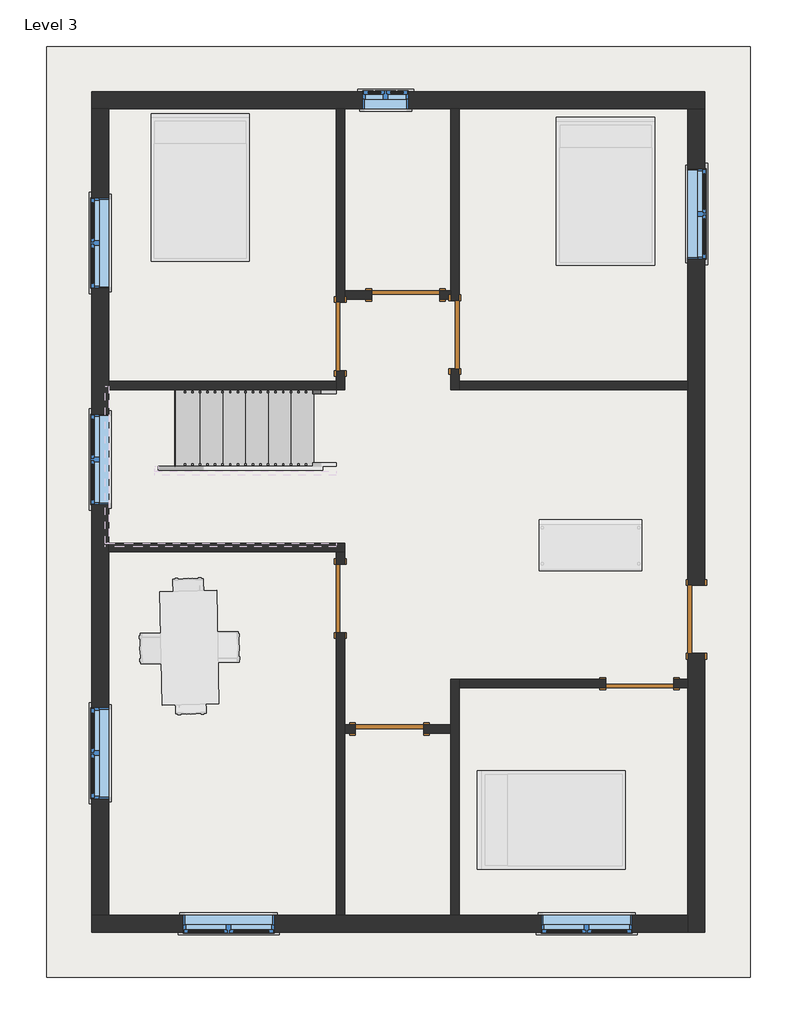
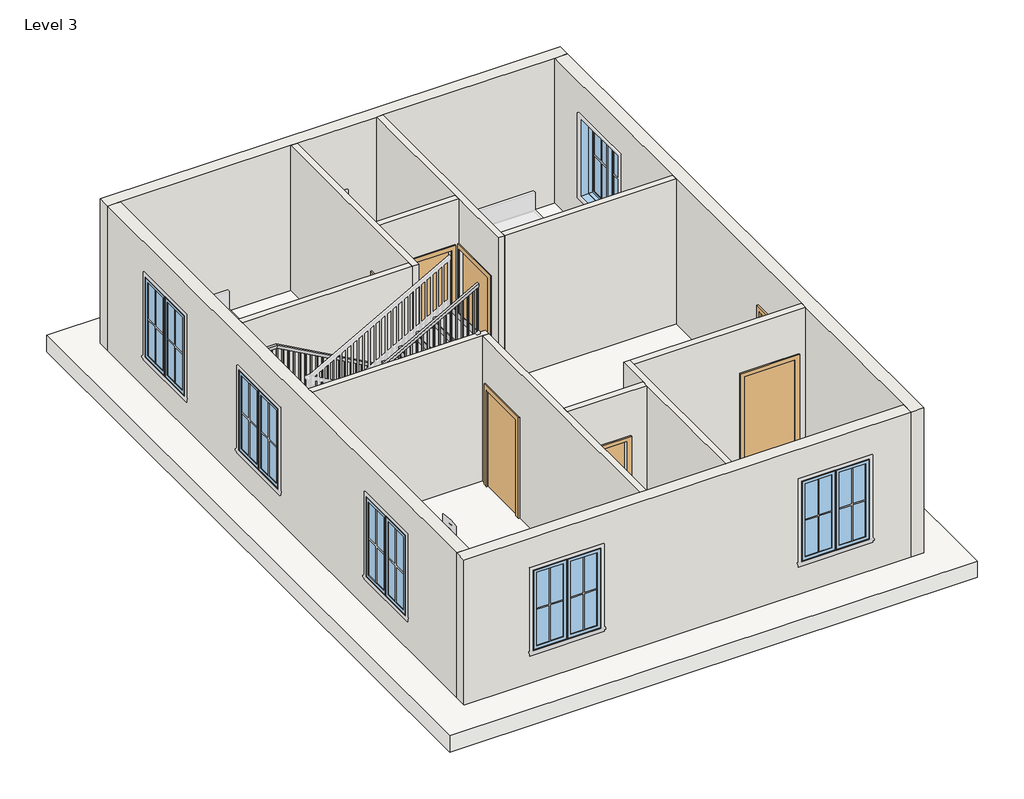
# One storey, part 1 of 2: 14 walls, 7 doors, 7 windows, 1 railing, 1 roof, 1 stair flight.
"""IFC4 building model written with IfcOpenShell, lengths in millimetres."""

from ifc_helpers import new_model, si_unit, frame, origin, place, context, project, spatial, polyline, outline, extrude, faceted_brep, transform, mapped, element, save
from components import door_e5f9f3c4, door_305aa2a5, door_a90ba1ad, stair_flight_67f7f0a7, window_c417fced, window_8377141f

model = new_model("IFC4")

# Units and contexts
model_context = context("Model", 3, world=origin())
ifc_project = project(units=[si_unit("LENGTHUNIT", "METRE", prefix="MILLI")], contexts=[model_context])

# Site, building, storey
site = spatial("IfcSite", under=ifc_project)
building = spatial("IfcBuilding", under=site)
storey = spatial("IfcBuildingStorey", under=building, Name="Level 3", Elevation=6096.0)

# Doors
placement = place(None, origin())
door_shape = door_e5f9f3c4(model_context)
element("IfcDoor", 1, ObjectType="Single-Flush : 36\" x 84\"", at=placement, inside=storey, context=model_context, shape_type="MappedRepresentation", body=[
    mapped(door_shape, transform((5226.05, 11245.85, 6096.0), x_axis=(1.0, 0.0, 0.0), y_axis=(0.0, 1.0, 0.0), z_axis=(0.0, 0.0, 1.0))),
])
element("IfcDoor", 2, ObjectType="Single-Flush : 36\" x 84\"", at=placement, inside=storey, context=model_context, shape_type="MappedRepresentation", body=[
    mapped(door_shape, transform((5886.45, 10712.45, 6096.0), x_axis=(0.0, -1.0, 0.0), y_axis=(1.0, 0.0, 0.0), z_axis=(0.0, 0.0, 1.0))),
])
door_2_shape = door_305aa2a5(model_context)
element("IfcDoor", 3, ObjectType="Single-Flush : 36\" x 84\"", at=placement, inside=storey, context=model_context, shape_type="MappedRepresentation", body=[
    mapped(door_2_shape, transform((4349.75, 10687.05, 6096.0), x_axis=(0.0, -1.0, 0.0), y_axis=(1.0, 0.0, 0.0), z_axis=(0.0, 0.0, 1.0))),
])
element("IfcDoor", 4, ObjectType="Single-Flush : 36\" x 84\"", at=placement, inside=storey, context=model_context, shape_type="MappedRepresentation", body=[
    mapped(door_2_shape, transform((8369.3, 6026.15, 6096.0), x_axis=(1.0, 0.0, 0.0), y_axis=(0.0, 1.0, 0.0), z_axis=(0.0, 0.0, 1.0))),
])
element("IfcDoor", 5, ObjectType="Single-Flush : 36\" x 84\"", at=placement, inside=storey, context=model_context, shape_type="MappedRepresentation", body=[
    mapped(door_2_shape, transform((5010.15, 5416.55, 6096.0), x_axis=(-1.0, 0.0, 0.0), y_axis=(0.0, -1.0, 0.0), z_axis=(0.0, 0.0, 1.0))),
])
element("IfcDoor", 6, ObjectType="Single-Flush : 36\" x 84\"", at=placement, inside=storey, context=model_context, shape_type="MappedRepresentation", body=[
    mapped(door_2_shape, transform((4349.75, 7169.15, 6096.0), x_axis=(0.0, -1.0, 0.0), y_axis=(1.0, 0.0, 0.0), z_axis=(0.0, 0.0, 1.0))),
])
door_3_shape = door_a90ba1ad(model_context)
element("IfcDoor", 7, ObjectType="Single-Flush : 36\" x 84\"", at=placement, inside=storey, context=model_context, shape_type="MappedRepresentation", body=[
    mapped(door_3_shape, transform((9131.3, 6889.75, 6096.0), x_axis=(0.0, -1.0, 0.0), y_axis=(1.0, 0.0, 0.0), z_axis=(0.0, 0.0, 1.0))),
])

# Railing
element("IfcRailing", 8, ObjectType="Handrail - Rectangular", at=placement, inside=storey, context=model_context, shape_type="SolidModel", body=[
    faceted_brep([(4295.1355783, 9918.7, 7179.7333333), (4295.1355783, 9918.7, 7121.620221), (4295.1355783, 9969.5, 7121.620221), (4295.1355783, 9969.5, 7179.7333333), (1856.7355783, 9918.7, 8534.4), (1843.5719761, 9918.7, 8483.6), (1843.5719761, 9969.5, 8483.6), (1856.7355783, 9969.5, 8534.4), (1295.4, 9918.7, 8534.4), (1295.4, 9918.7, 8483.6), (1244.6, 9969.5, 8483.6), (1244.6, 9969.5, 8534.4), (1295.4, 7962.9, 8534.4), (1295.4, 7962.9, 8483.6), (1244.6, 7912.1, 8483.6), (1244.6, 7912.1, 8534.4), (1551.9355783, 7962.9, 8534.4), (1565.0991806, 7962.9, 8483.6), (1565.0991806, 7912.1, 8483.6), (1551.9355783, 7912.1, 8534.4), (4295.1355783, 7962.9, 10058.4), (4295.1355783, 7912.1, 10058.4), (4295.1355783, 7912.1, 10000.2868876), (4295.1355783, 7962.9, 10000.2868876)], [[[0, 1, 2, 3]], [[1, 0, 4, 5]], [[2, 1, 5, 6]], [[3, 2, 6, 7]], [[0, 3, 7, 4]], [[5, 4, 8, 9]], [[6, 5, 9, 10]], [[7, 6, 10, 11]], [[4, 7, 11, 8]], [[9, 8, 12, 13]], [[10, 9, 13, 14]], [[11, 10, 14, 15]], [[8, 11, 15, 12]], [[13, 12, 16, 17]], [[14, 13, 17, 18]], [[15, 14, 18, 19]], [[12, 15, 19, 16]], [[20, 21, 22, 23]], [[17, 16, 20, 23]], [[18, 17, 23, 22]], [[19, 18, 22, 21]], [[16, 19, 21, 20]]]),
    extrude(outline(polyline([(9961.8365664, 4225.925), (9951.253233, 4206.875), (8974.6666667, 4206.875), (8974.6666667, 4225.925), (9961.8365664, 4225.925)])), frame((0.0, 7927.975, 0.0), z_axis=(0.0, 1.0, 0.0), x_axis=(0.0, 0.0, 1.0)), (0.0, 0.0, 1.0), 19.05),
    extrude(outline(polyline([(9905.3921219, 4124.325), (9894.8087886, 4105.275), (8974.6666667, 4105.275), (8974.6666667, 4124.325), (9905.3921219, 4124.325)])), frame((0.0, 7927.975, 0.0), z_axis=(0.0, 1.0, 0.0), x_axis=(0.0, 0.0, 1.0)), (0.0, 0.0, 1.0), 19.05),
    extrude(outline(polyline([(9848.9476775, 4022.725), (9838.3643441, 4003.675), (8974.6666667, 4003.675), (8974.6666667, 4022.725), (9848.9476775, 4022.725)])), frame((0.0, 7927.975, 0.0), z_axis=(0.0, 1.0, 0.0), x_axis=(0.0, 0.0, 1.0)), (0.0, 0.0, 1.0), 19.05),
    extrude(outline(polyline([(9792.503233, 3921.125), (9781.9198997, 3902.075), (8805.3333333, 3902.075), (8805.3333333, 3921.125), (9792.503233, 3921.125)])), frame((0.0, 7927.975, 0.0), z_axis=(0.0, 1.0, 0.0), x_axis=(0.0, 0.0, 1.0)), (0.0, 0.0, 1.0), 19.05),
    extrude(outline(polyline([(9736.0587886, 3819.525), (9725.4754552, 3800.475), (8805.3333333, 3800.475), (8805.3333333, 3819.525), (9736.0587886, 3819.525)])), frame((0.0, 7927.975, 0.0), z_axis=(0.0, 1.0, 0.0), x_axis=(0.0, 0.0, 1.0)), (0.0, 0.0, 1.0), 19.05),
    extrude(outline(polyline([(9679.6143441, 3717.925), (9669.0310108, 3698.875), (8805.3333333, 3698.875), (8805.3333333, 3717.925), (9679.6143441, 3717.925)])), frame((0.0, 7927.975, 0.0), z_axis=(0.0, 1.0, 0.0), x_axis=(0.0, 0.0, 1.0)), (0.0, 0.0, 1.0), 19.05),
    extrude(outline(polyline([(9623.1698997, 3616.325), (9612.5865664, 3597.275), (8636.0, 3597.275), (8636.0, 3616.325), (9623.1698997, 3616.325)])), frame((0.0, 7927.975, 0.0), z_axis=(0.0, 1.0, 0.0), x_axis=(0.0, 0.0, 1.0)), (0.0, 0.0, 1.0), 19.05),
    extrude(outline(polyline([(9566.7254552, 3514.725), (9556.1421219, 3495.675), (8636.0, 3495.675), (8636.0, 3514.725), (9566.7254552, 3514.725)])), frame((0.0, 7927.975, 0.0), z_axis=(0.0, 1.0, 0.0), x_axis=(0.0, 0.0, 1.0)), (0.0, 0.0, 1.0), 19.05),
    extrude(outline(polyline([(9510.2810108, 3413.125), (9499.6976775, 3394.075), (8636.0, 3394.075), (8636.0, 3413.125), (9510.2810108, 3413.125)])), frame((0.0, 7927.975, 0.0), z_axis=(0.0, 1.0, 0.0), x_axis=(0.0, 0.0, 1.0)), (0.0, 0.0, 1.0), 19.05),
    extrude(outline(polyline([(9453.8365664, 3311.525), (9443.253233, 3292.475), (8466.6666667, 3292.475), (8466.6666667, 3311.525), (9453.8365664, 3311.525)])), frame((0.0, 7927.975, 0.0), z_axis=(0.0, 1.0, 0.0), x_axis=(0.0, 0.0, 1.0)), (0.0, 0.0, 1.0), 19.05),
    extrude(outline(polyline([(9397.3921219, 3209.925), (9386.8087886, 3190.875), (8466.6666667, 3190.875), (8466.6666667, 3209.925), (9397.3921219, 3209.925)])), frame((0.0, 7927.975, 0.0), z_axis=(0.0, 1.0, 0.0), x_axis=(0.0, 0.0, 1.0)), (0.0, 0.0, 1.0), 19.05),
    extrude(outline(polyline([(9340.9476775, 3108.325), (9330.3643441, 3089.275), (8466.6666667, 3089.275), (8466.6666667, 3108.325), (9340.9476775, 3108.325)])), frame((0.0, 7927.975, 0.0), z_axis=(0.0, 1.0, 0.0), x_axis=(0.0, 0.0, 1.0)), (0.0, 0.0, 1.0), 19.05),
    extrude(outline(polyline([(9284.503233, 3006.725), (9273.9198997, 2987.675), (8297.3333333, 2987.675), (8297.3333333, 3006.725), (9284.503233, 3006.725)])), frame((0.0, 7927.975, 0.0), z_axis=(0.0, 1.0, 0.0), x_axis=(0.0, 0.0, 1.0)), (0.0, 0.0, 1.0), 19.05),
    extrude(outline(polyline([(9228.0587886, 2905.125), (9217.4754552, 2886.075), (8297.3333333, 2886.075), (8297.3333333, 2905.125), (9228.0587886, 2905.125)])), frame((0.0, 7927.975, 0.0), z_axis=(0.0, 1.0, 0.0), x_axis=(0.0, 0.0, 1.0)), (0.0, 0.0, 1.0), 19.05),
    extrude(outline(polyline([(9171.6143441, 2803.525), (9161.0310108, 2784.475), (8297.3333333, 2784.475), (8297.3333333, 2803.525), (9171.6143441, 2803.525)])), frame((0.0, 7927.975, 0.0), z_axis=(0.0, 1.0, 0.0), x_axis=(0.0, 0.0, 1.0)), (0.0, 0.0, 1.0), 19.05),
    extrude(outline(polyline([(9115.1698997, 2701.925), (9104.5865664, 2682.875), (8128.0, 2682.875), (8128.0, 2701.925), (9115.1698997, 2701.925)])), frame((0.0, 7927.975, 0.0), z_axis=(0.0, 1.0, 0.0), x_axis=(0.0, 0.0, 1.0)), (0.0, 0.0, 1.0), 19.05),
    extrude(outline(polyline([(9058.7254552, 2600.325), (9048.1421219, 2581.275), (8128.0, 2581.275), (8128.0, 2600.325), (9058.7254552, 2600.325)])), frame((0.0, 7927.975, 0.0), z_axis=(0.0, 1.0, 0.0), x_axis=(0.0, 0.0, 1.0)), (0.0, 0.0, 1.0), 19.05),
    extrude(outline(polyline([(9002.2810108, 2498.725), (8991.6976775, 2479.675), (8128.0, 2479.675), (8128.0, 2498.725), (9002.2810108, 2498.725)])), frame((0.0, 7927.975, 0.0), z_axis=(0.0, 1.0, 0.0), x_axis=(0.0, 0.0, 1.0)), (0.0, 0.0, 1.0), 19.05),
    extrude(outline(polyline([(8945.8365664, 2397.125), (8935.253233, 2378.075), (7958.6666667, 2378.075), (7958.6666667, 2397.125), (8945.8365664, 2397.125)])), frame((0.0, 7927.975, 0.0), z_axis=(0.0, 1.0, 0.0), x_axis=(0.0, 0.0, 1.0)), (0.0, 0.0, 1.0), 19.05),
    extrude(outline(polyline([(8889.3921219, 2295.525), (8878.8087886, 2276.475), (7958.6666667, 2276.475), (7958.6666667, 2295.525), (8889.3921219, 2295.525)])), frame((0.0, 7927.975, 0.0), z_axis=(0.0, 1.0, 0.0), x_axis=(0.0, 0.0, 1.0)), (0.0, 0.0, 1.0), 19.05),
    extrude(outline(polyline([(8832.9476775, 2193.925), (8822.3643441, 2174.875), (7958.6666667, 2174.875), (7958.6666667, 2193.925), (8832.9476775, 2193.925)])), frame((0.0, 7927.975, 0.0), z_axis=(0.0, 1.0, 0.0), x_axis=(0.0, 0.0, 1.0)), (0.0, 0.0, 1.0), 19.05),
    extrude(outline(polyline([(8776.503233, 2092.325), (8765.9198997, 2073.275), (7789.3333333, 2073.275), (7789.3333333, 2092.325), (8776.503233, 2092.325)])), frame((0.0, 7927.975, 0.0), z_axis=(0.0, 1.0, 0.0), x_axis=(0.0, 0.0, 1.0)), (0.0, 0.0, 1.0), 19.05),
    extrude(outline(polyline([(8720.0587886, 1990.725), (8709.4754552, 1971.675), (7789.3333333, 1971.675), (7789.3333333, 1990.725), (8720.0587886, 1990.725)])), frame((0.0, 7927.975, 0.0), z_axis=(0.0, 1.0, 0.0), x_axis=(0.0, 0.0, 1.0)), (0.0, 0.0, 1.0), 19.05),
    extrude(outline(polyline([(8663.6143441, 1889.125), (8653.0310108, 1870.075), (7789.3333333, 1870.075), (7789.3333333, 1889.125), (8663.6143441, 1889.125)])), frame((0.0, 7927.975, 0.0), z_axis=(0.0, 1.0, 0.0), x_axis=(0.0, 0.0, 1.0)), (0.0, 0.0, 1.0), 19.05),
    extrude(outline(polyline([(8607.1698997, 1787.525), (8596.5865664, 1768.475), (7620.0, 1768.475), (7620.0, 1787.525), (8607.1698997, 1787.525)])), frame((0.0, 7927.975, 0.0), z_axis=(0.0, 1.0, 0.0), x_axis=(0.0, 0.0, 1.0)), (0.0, 0.0, 1.0), 19.05),
    extrude(outline(polyline([(8550.7254552, 1685.925), (8540.1421219, 1666.875), (7620.0, 1666.875), (7620.0, 1685.925), (8550.7254552, 1685.925)])), frame((0.0, 7927.975, 0.0), z_axis=(0.0, 1.0, 0.0), x_axis=(0.0, 0.0, 1.0)), (0.0, 0.0, 1.0), 19.05),
    extrude(outline(polyline([(8494.2810108, 1584.325), (8483.6976775, 1565.275), (7620.0, 1565.275), (7620.0, 1584.325), (8494.2810108, 1584.325)])), frame((0.0, 7927.975, 0.0), z_axis=(0.0, 1.0, 0.0), x_axis=(0.0, 0.0, 1.0)), (0.0, 0.0, 1.0), 19.05),
    extrude(outline(polyline([(1463.675, 7927.975), (1463.675, 7947.025), (1482.725, 7947.025), (1482.725, 7927.975), (1463.675, 7927.975)])), frame((0.0, 0.0, 7620.0), z_axis=(0.0, 0.0, 1.0), x_axis=(1.0, 0.0, 0.0)), (0.0, 0.0, 1.0), 863.6),
    extrude(outline(polyline([(1362.075, 7927.975), (1362.075, 7947.025), (1381.125, 7947.025), (1381.125, 7927.975), (1362.075, 7927.975)])), frame((0.0, 0.0, 7620.0), z_axis=(0.0, 0.0, 1.0), x_axis=(1.0, 0.0, 0.0)), (0.0, 0.0, 1.0), 863.6),
    extrude(outline(polyline([(1260.475, 8023.225), (1279.525, 8023.225), (1279.525, 8004.175), (1260.475, 8004.175), (1260.475, 8023.225)])), frame((0.0, 0.0, 7620.0), z_axis=(0.0, 0.0, 1.0), x_axis=(1.0, 0.0, 0.0)), (0.0, 0.0, 1.0), 863.6),
    extrude(outline(polyline([(1260.475, 8124.825), (1279.525, 8124.825), (1279.525, 8105.775), (1260.475, 8105.775), (1260.475, 8124.825)])), frame((0.0, 0.0, 7620.0), z_axis=(0.0, 0.0, 1.0), x_axis=(1.0, 0.0, 0.0)), (0.0, 0.0, 1.0), 863.6),
    extrude(outline(polyline([(1260.475, 8226.425), (1279.525, 8226.425), (1279.525, 8207.375), (1260.475, 8207.375), (1260.475, 8226.425)])), frame((0.0, 0.0, 7620.0), z_axis=(0.0, 0.0, 1.0), x_axis=(1.0, 0.0, 0.0)), (0.0, 0.0, 1.0), 863.6),
    extrude(outline(polyline([(1260.475, 8328.025), (1279.525, 8328.025), (1279.525, 8308.975), (1260.475, 8308.975), (1260.475, 8328.025)])), frame((0.0, 0.0, 7620.0), z_axis=(0.0, 0.0, 1.0), x_axis=(1.0, 0.0, 0.0)), (0.0, 0.0, 1.0), 863.6),
    extrude(outline(polyline([(1260.475, 8429.625), (1279.525, 8429.625), (1279.525, 8410.575), (1260.475, 8410.575), (1260.475, 8429.625)])), frame((0.0, 0.0, 7620.0), z_axis=(0.0, 0.0, 1.0), x_axis=(1.0, 0.0, 0.0)), (0.0, 0.0, 1.0), 863.6),
    extrude(outline(polyline([(1260.475, 8531.225), (1279.525, 8531.225), (1279.525, 8512.175), (1260.475, 8512.175), (1260.475, 8531.225)])), frame((0.0, 0.0, 7620.0), z_axis=(0.0, 0.0, 1.0), x_axis=(1.0, 0.0, 0.0)), (0.0, 0.0, 1.0), 863.6),
    extrude(outline(polyline([(1260.475, 8632.825), (1279.525, 8632.825), (1279.525, 8613.775), (1260.475, 8613.775), (1260.475, 8632.825)])), frame((0.0, 0.0, 7620.0), z_axis=(0.0, 0.0, 1.0), x_axis=(1.0, 0.0, 0.0)), (0.0, 0.0, 1.0), 863.6),
    extrude(outline(polyline([(1260.475, 8734.425), (1279.525, 8734.425), (1279.525, 8715.375), (1260.475, 8715.375), (1260.475, 8734.425)])), frame((0.0, 0.0, 7620.0), z_axis=(0.0, 0.0, 1.0), x_axis=(1.0, 0.0, 0.0)), (0.0, 0.0, 1.0), 863.6),
    extrude(outline(polyline([(1260.475, 8836.025), (1279.525, 8836.025), (1279.525, 8816.975), (1260.475, 8816.975), (1260.475, 8836.025)])), frame((0.0, 0.0, 7620.0), z_axis=(0.0, 0.0, 1.0), x_axis=(1.0, 0.0, 0.0)), (0.0, 0.0, 1.0), 863.6),
    extrude(outline(polyline([(1260.475, 8937.625), (1279.525, 8937.625), (1279.525, 8918.575), (1260.475, 8918.575), (1260.475, 8937.625)])), frame((0.0, 0.0, 7620.0), z_axis=(0.0, 0.0, 1.0), x_axis=(1.0, 0.0, 0.0)), (0.0, 0.0, 1.0), 863.6),
    extrude(outline(polyline([(1260.475, 9039.225), (1279.525, 9039.225), (1279.525, 9020.175), (1260.475, 9020.175), (1260.475, 9039.225)])), frame((0.0, 0.0, 7620.0), z_axis=(0.0, 0.0, 1.0), x_axis=(1.0, 0.0, 0.0)), (0.0, 0.0, 1.0), 863.6),
    extrude(outline(polyline([(1260.475, 9140.825), (1279.525, 9140.825), (1279.525, 9121.775), (1260.475, 9121.775), (1260.475, 9140.825)])), frame((0.0, 0.0, 7620.0), z_axis=(0.0, 0.0, 1.0), x_axis=(1.0, 0.0, 0.0)), (0.0, 0.0, 1.0), 863.6),
    extrude(outline(polyline([(1260.475, 9242.425), (1279.525, 9242.425), (1279.525, 9223.375), (1260.475, 9223.375), (1260.475, 9242.425)])), frame((0.0, 0.0, 7620.0), z_axis=(0.0, 0.0, 1.0), x_axis=(1.0, 0.0, 0.0)), (0.0, 0.0, 1.0), 863.6),
    extrude(outline(polyline([(1260.475, 9344.025), (1279.525, 9344.025), (1279.525, 9324.975), (1260.475, 9324.975), (1260.475, 9344.025)])), frame((0.0, 0.0, 7620.0), z_axis=(0.0, 0.0, 1.0), x_axis=(1.0, 0.0, 0.0)), (0.0, 0.0, 1.0), 863.6),
    extrude(outline(polyline([(1260.475, 9445.625), (1279.525, 9445.625), (1279.525, 9426.575), (1260.475, 9426.575), (1260.475, 9445.625)])), frame((0.0, 0.0, 7620.0), z_axis=(0.0, 0.0, 1.0), x_axis=(1.0, 0.0, 0.0)), (0.0, 0.0, 1.0), 863.6),
    extrude(outline(polyline([(1260.475, 9547.225), (1279.525, 9547.225), (1279.525, 9528.175), (1260.475, 9528.175), (1260.475, 9547.225)])), frame((0.0, 0.0, 7620.0), z_axis=(0.0, 0.0, 1.0), x_axis=(1.0, 0.0, 0.0)), (0.0, 0.0, 1.0), 863.6),
    extrude(outline(polyline([(1260.475, 9648.825), (1279.525, 9648.825), (1279.525, 9629.775), (1260.475, 9629.775), (1260.475, 9648.825)])), frame((0.0, 0.0, 7620.0), z_axis=(0.0, 0.0, 1.0), x_axis=(1.0, 0.0, 0.0)), (0.0, 0.0, 1.0), 863.6),
    extrude(outline(polyline([(1260.475, 9750.425), (1279.525, 9750.425), (1279.525, 9731.375), (1260.475, 9731.375), (1260.475, 9750.425)])), frame((0.0, 0.0, 7620.0), z_axis=(0.0, 0.0, 1.0), x_axis=(1.0, 0.0, 0.0)), (0.0, 0.0, 1.0), 863.6),
    extrude(outline(polyline([(1260.475, 9852.025), (1279.525, 9852.025), (1279.525, 9832.975), (1260.475, 9832.975), (1260.475, 9852.025)])), frame((0.0, 0.0, 7620.0), z_axis=(0.0, 0.0, 1.0), x_axis=(1.0, 0.0, 0.0)), (0.0, 0.0, 1.0), 863.6),
    extrude(outline(polyline([(1358.2605783, 9953.625), (1358.2605783, 9934.575), (1339.2105783, 9934.575), (1339.2105783, 9953.625), (1358.2605783, 9953.625)])), frame((0.0, 0.0, 7620.0), z_axis=(0.0, 0.0, 1.0), x_axis=(1.0, 0.0, 0.0)), (0.0, 0.0, 1.0), 863.6),
    extrude(outline(polyline([(1459.8605783, 9953.625), (1459.8605783, 9934.575), (1440.8105783, 9934.575), (1440.8105783, 9953.625), (1459.8605783, 9953.625)])), frame((0.0, 0.0, 7620.0), z_axis=(0.0, 0.0, 1.0), x_axis=(1.0, 0.0, 0.0)), (0.0, 0.0, 1.0), 863.6),
    extrude(outline(polyline([(1561.4605783, 9953.625), (1561.4605783, 9934.575), (1542.4105783, 9934.575), (1542.4105783, 9953.625), (1561.4605783, 9953.625)])), frame((0.0, 0.0, 7620.0), z_axis=(0.0, 0.0, 1.0), x_axis=(1.0, 0.0, 0.0)), (0.0, 0.0, 1.0), 863.6),
    extrude(outline(polyline([(1663.0605783, 9953.625), (1663.0605783, 9934.575), (1644.0105783, 9934.575), (1644.0105783, 9953.625), (1663.0605783, 9953.625)])), frame((0.0, 0.0, 7620.0), z_axis=(0.0, 0.0, 1.0), x_axis=(1.0, 0.0, 0.0)), (0.0, 0.0, 1.0), 863.6),
    extrude(outline(polyline([(1764.6605783, 9953.625), (1764.6605783, 9934.575), (1745.6105783, 9934.575), (1745.6105783, 9953.625), (1764.6605783, 9953.625)])), frame((0.0, 0.0, 7620.0), z_axis=(0.0, 0.0, 1.0), x_axis=(1.0, 0.0, 0.0)), (0.0, 0.0, 1.0), 863.6),
    extrude(outline(polyline([(8470.995221, 1866.2605783), (8481.5785543, 1847.2105783), (7620.0, 1847.2105783), (7620.0, 1866.2605783), (8470.995221, 1866.2605783)])), frame((0.0, 9934.575, 0.0), z_axis=(0.0, 1.0, 0.0), x_axis=(0.0, 0.0, 1.0)), (0.0, 0.0, 1.0), 19.05),
    extrude(outline(polyline([(8414.5507765, 1967.8605783), (8425.1341099, 1948.8105783), (7450.6666667, 1948.8105783), (7450.6666667, 1967.8605783), (8414.5507765, 1967.8605783)])), frame((0.0, 9934.575, 0.0), z_axis=(0.0, 1.0, 0.0), x_axis=(0.0, 0.0, 1.0)), (0.0, 0.0, 1.0), 19.05),
    extrude(outline(polyline([(8358.1063321, 2069.4605783), (8368.6896654, 2050.4105783), (7450.6666667, 2050.4105783), (7450.6666667, 2069.4605783), (8358.1063321, 2069.4605783)])), frame((0.0, 9934.575, 0.0), z_axis=(0.0, 1.0, 0.0), x_axis=(0.0, 0.0, 1.0)), (0.0, 0.0, 1.0), 19.05),
    extrude(outline(polyline([(8301.6618876, 2171.0605783), (8312.245221, 2152.0105783), (7450.6666667, 2152.0105783), (7450.6666667, 2171.0605783), (8301.6618876, 2171.0605783)])), frame((0.0, 9934.575, 0.0), z_axis=(0.0, 1.0, 0.0), x_axis=(0.0, 0.0, 1.0)), (0.0, 0.0, 1.0), 19.05),
    extrude(outline(polyline([(8245.2174432, 2272.6605783), (8255.8007765, 2253.6105783), (7281.3333333, 2253.6105783), (7281.3333333, 2272.6605783), (8245.2174432, 2272.6605783)])), frame((0.0, 9934.575, 0.0), z_axis=(0.0, 1.0, 0.0), x_axis=(0.0, 0.0, 1.0)), (0.0, 0.0, 1.0), 19.05),
    extrude(outline(polyline([(8188.7729988, 2374.2605783), (8199.3563321, 2355.2105783), (7281.3333333, 2355.2105783), (7281.3333333, 2374.2605783), (8188.7729988, 2374.2605783)])), frame((0.0, 9934.575, 0.0), z_axis=(0.0, 1.0, 0.0), x_axis=(0.0, 0.0, 1.0)), (0.0, 0.0, 1.0), 19.05),
    extrude(outline(polyline([(8132.3285543, 2475.8605783), (8142.9118876, 2456.8105783), (7281.3333333, 2456.8105783), (7281.3333333, 2475.8605783), (8132.3285543, 2475.8605783)])), frame((0.0, 9934.575, 0.0), z_axis=(0.0, 1.0, 0.0), x_axis=(0.0, 0.0, 1.0)), (0.0, 0.0, 1.0), 19.05),
    extrude(outline(polyline([(8075.8841099, 2577.4605783), (8086.4674432, 2558.4105783), (7112.0, 2558.4105783), (7112.0, 2577.4605783), (8075.8841099, 2577.4605783)])), frame((0.0, 9934.575, 0.0), z_axis=(0.0, 1.0, 0.0), x_axis=(0.0, 0.0, 1.0)), (0.0, 0.0, 1.0), 19.05),
    extrude(outline(polyline([(8019.4396654, 2679.0605783), (8030.0229988, 2660.0105783), (7112.0, 2660.0105783), (7112.0, 2679.0605783), (8019.4396654, 2679.0605783)])), frame((0.0, 9934.575, 0.0), z_axis=(0.0, 1.0, 0.0), x_axis=(0.0, 0.0, 1.0)), (0.0, 0.0, 1.0), 19.05),
    extrude(outline(polyline([(7962.995221, 2780.6605783), (7973.5785543, 2761.6105783), (7112.0, 2761.6105783), (7112.0, 2780.6605783), (7962.995221, 2780.6605783)])), frame((0.0, 9934.575, 0.0), z_axis=(0.0, 1.0, 0.0), x_axis=(0.0, 0.0, 1.0)), (0.0, 0.0, 1.0), 19.05),
    extrude(outline(polyline([(7906.5507765, 2882.2605783), (7917.1341099, 2863.2105783), (6942.6666667, 2863.2105783), (6942.6666667, 2882.2605783), (7906.5507765, 2882.2605783)])), frame((0.0, 9934.575, 0.0), z_axis=(0.0, 1.0, 0.0), x_axis=(0.0, 0.0, 1.0)), (0.0, 0.0, 1.0), 19.05),
    extrude(outline(polyline([(7850.1063321, 2983.8605783), (7860.6896654, 2964.8105783), (6942.6666667, 2964.8105783), (6942.6666667, 2983.8605783), (7850.1063321, 2983.8605783)])), frame((0.0, 9934.575, 0.0), z_axis=(0.0, 1.0, 0.0), x_axis=(0.0, 0.0, 1.0)), (0.0, 0.0, 1.0), 19.05),
    extrude(outline(polyline([(7793.6618876, 3085.4605783), (7804.245221, 3066.4105783), (6942.6666667, 3066.4105783), (6942.6666667, 3085.4605783), (7793.6618876, 3085.4605783)])), frame((0.0, 9934.575, 0.0), z_axis=(0.0, 1.0, 0.0), x_axis=(0.0, 0.0, 1.0)), (0.0, 0.0, 1.0), 19.05),
    extrude(outline(polyline([(7737.2174432, 3187.0605783), (7747.8007765, 3168.0105783), (6773.3333333, 3168.0105783), (6773.3333333, 3187.0605783), (7737.2174432, 3187.0605783)])), frame((0.0, 9934.575, 0.0), z_axis=(0.0, 1.0, 0.0), x_axis=(0.0, 0.0, 1.0)), (0.0, 0.0, 1.0), 19.05),
    extrude(outline(polyline([(7680.7729988, 3288.6605783), (7691.3563321, 3269.6105783), (6773.3333333, 3269.6105783), (6773.3333333, 3288.6605783), (7680.7729988, 3288.6605783)])), frame((0.0, 9934.575, 0.0), z_axis=(0.0, 1.0, 0.0), x_axis=(0.0, 0.0, 1.0)), (0.0, 0.0, 1.0), 19.05),
    extrude(outline(polyline([(7624.3285543, 3390.2605783), (7634.9118876, 3371.2105783), (6773.3333333, 3371.2105783), (6773.3333333, 3390.2605783), (7624.3285543, 3390.2605783)])), frame((0.0, 9934.575, 0.0), z_axis=(0.0, 1.0, 0.0), x_axis=(0.0, 0.0, 1.0)), (0.0, 0.0, 1.0), 19.05),
    extrude(outline(polyline([(7567.8841099, 3491.8605783), (7578.4674432, 3472.8105783), (6604.0, 3472.8105783), (6604.0, 3491.8605783), (7567.8841099, 3491.8605783)])), frame((0.0, 9934.575, 0.0), z_axis=(0.0, 1.0, 0.0), x_axis=(0.0, 0.0, 1.0)), (0.0, 0.0, 1.0), 19.05),
    extrude(outline(polyline([(7511.4396654, 3593.4605783), (7522.0229988, 3574.4105783), (6604.0, 3574.4105783), (6604.0, 3593.4605783), (7511.4396654, 3593.4605783)])), frame((0.0, 9934.575, 0.0), z_axis=(0.0, 1.0, 0.0), x_axis=(0.0, 0.0, 1.0)), (0.0, 0.0, 1.0), 19.05),
    extrude(outline(polyline([(7454.995221, 3695.0605783), (7465.5785543, 3676.0105783), (6604.0, 3676.0105783), (6604.0, 3695.0605783), (7454.995221, 3695.0605783)])), frame((0.0, 9934.575, 0.0), z_axis=(0.0, 1.0, 0.0), x_axis=(0.0, 0.0, 1.0)), (0.0, 0.0, 1.0), 19.05),
    extrude(outline(polyline([(7398.5507765, 3796.6605783), (7409.1341099, 3777.6105783), (6434.6666667, 3777.6105783), (6434.6666667, 3796.6605783), (7398.5507765, 3796.6605783)])), frame((0.0, 9934.575, 0.0), z_axis=(0.0, 1.0, 0.0), x_axis=(0.0, 0.0, 1.0)), (0.0, 0.0, 1.0), 19.05),
    extrude(outline(polyline([(7342.1063321, 3898.2605783), (7352.6896654, 3879.2105783), (6434.6666667, 3879.2105783), (6434.6666667, 3898.2605783), (7342.1063321, 3898.2605783)])), frame((0.0, 9934.575, 0.0), z_axis=(0.0, 1.0, 0.0), x_axis=(0.0, 0.0, 1.0)), (0.0, 0.0, 1.0), 19.05),
    extrude(outline(polyline([(7285.6618876, 3999.8605783), (7296.245221, 3980.8105783), (6434.6666667, 3980.8105783), (6434.6666667, 3999.8605783), (7285.6618876, 3999.8605783)])), frame((0.0, 9934.575, 0.0), z_axis=(0.0, 1.0, 0.0), x_axis=(0.0, 0.0, 1.0)), (0.0, 0.0, 1.0), 19.05),
    extrude(outline(polyline([(7229.2174432, 4101.4605783), (7239.8007765, 4082.4105783), (6265.3333333, 4082.4105783), (6265.3333333, 4101.4605783), (7229.2174432, 4101.4605783)])), frame((0.0, 9934.575, 0.0), z_axis=(0.0, 1.0, 0.0), x_axis=(0.0, 0.0, 1.0)), (0.0, 0.0, 1.0), 19.05),
    extrude(outline(polyline([(7172.7729988, 4203.0605783), (7183.3563321, 4184.0105783), (6265.3333333, 4184.0105783), (6265.3333333, 4203.0605783), (7172.7729988, 4203.0605783)])), frame((0.0, 9934.575, 0.0), z_axis=(0.0, 1.0, 0.0), x_axis=(0.0, 0.0, 1.0)), (0.0, 0.0, 1.0), 19.05),
    extrude(outline(polyline([(1260.475, 7947.025), (1279.525, 7947.025), (1279.525, 7927.975), (1260.475, 7927.975), (1260.475, 7947.025)])), frame((0.0, 0.0, 7620.0), z_axis=(0.0, 0.0, 1.0), x_axis=(1.0, 0.0, 0.0)), (0.0, 0.0, 1.0), 863.6),
    extrude(outline(polyline([(1279.525, 9953.625), (1279.525, 9934.575), (1260.475, 9934.575), (1260.475, 9953.625), (1279.525, 9953.625)])), frame((0.0, 0.0, 7620.0), z_axis=(0.0, 0.0, 1.0), x_axis=(1.0, 0.0, 0.0)), (0.0, 0.0, 1.0), 863.6),
    extrude(outline(polyline([(10000.2868876, 4295.1355783), (9989.7035543, 4276.0855783), (8974.6666667, 4276.0855783), (8974.6666667, 4295.1355783), (10000.2868876, 4295.1355783)])), frame((0.0, 7927.975, 0.0), z_axis=(0.0, 1.0, 0.0), x_axis=(0.0, 0.0, 1.0)), (0.0, 0.0, 1.0), 19.05),
    extrude(outline(polyline([(7121.620221, 4295.1355783), (7132.2035543, 4276.0855783), (6265.3333333, 4276.0855783), (6265.3333333, 4295.1355783), (7121.620221, 4295.1355783)])), frame((0.0, 9934.575, 0.0), z_axis=(0.0, 1.0, 0.0), x_axis=(0.0, 0.0, 1.0)), (0.0, 0.0, 1.0), 19.05),
])

# Roof
element("IfcRoof", 9, ObjectType="Generic - 12\"", at=placement, inside=storey, context=model_context, shape_type="SweptSolid", body=[
    extrude(outline(polyline([(406.4, 14579.6), (9855.2, 14579.6), (9855.2, 2082.8), (406.4, 2082.8), (406.4, 14579.6)])), frame((0.0, 0.0, 6096.0), z_axis=(0.0, 0.0, 1.0), x_axis=(1.0, 0.0, 0.0)), (0.0, 0.0, 1.0), 304.8),
])

# Stair flight
stair_flight_shape = stair_flight_67f7f0a7(model_context)
element("IfcStairFlight", 10, ObjectType="2\" Tread 1\" Nosing 1/4\" Riser", at=placement, inside=storey, context=model_context, shape_type="MappedRepresentation", body=[
    mapped(stair_flight_shape, transform((0.0, 0.0, 0.0), x_axis=(1.0, 0.0, 0.0), y_axis=(0.0, 1.0, 0.0), z_axis=(0.0, 0.0, 1.0))),
])

# Walls
element("IfcWall", 11, ObjectType="Generic - 5\"", at=placement, inside=storey, context=model_context, shape_type="Brep", body=[
    faceted_brep([(4292.6, 10229.85, 8229.6), (4292.6, 10229.85, 6096.0), (4292.6, 10083.8, 6096.0), (4292.6, 9969.5, 6096.0), (4292.6, 9969.5, 9144.0), (4292.6, 10083.8, 9144.0), (4292.6, 13741.4, 9144.0), (4292.6, 13741.4, 6096.0), (4292.6, 11144.25, 6096.0), (4292.6, 11144.25, 8229.6), (4406.9, 9969.5, 6096.0), (4406.9, 10229.85, 6096.0), (4406.9, 10229.85, 8229.6), (4406.9, 11144.25, 8229.6), (4406.9, 11144.25, 6096.0), (4406.9, 11188.7, 6096.0), (4406.9, 11303.0, 6096.0), (4406.9, 13741.4, 6096.0), (4406.9, 13741.4, 9144.0), (4406.9, 11303.0, 9144.0), (4406.9, 11188.7, 9144.0), (4406.9, 9969.5, 9144.0)], [[[0, 1, 2, 3, 4, 5, 6, 7, 8, 9]], [[10, 11, 12, 13, 14, 15, 16, 17, 18, 19, 20, 21]], [[8, 7, 17, 16, 15, 14]], [[3, 2, 1, 11, 10]], [[6, 5, 4, 21, 20, 19, 18]], [[7, 6, 18, 17]], [[4, 3, 10, 21]], [[12, 11, 1, 0]], [[13, 12, 0, 9]], [[14, 13, 9, 8]]]),
])
element("IfcWall", 12, ObjectType="Generic - 5\"", at=placement, inside=storey, context=model_context, shape_type="SweptSolid", body=[
    extrude(outline(polyline([(1244.6, 10083.8), (4292.6, 10083.8), (4292.6, 9969.5), (1244.6, 9969.5), (1244.6, 10083.8)])), frame((0.0, 0.0, 6096.0), z_axis=(0.0, 0.0, 1.0), x_axis=(1.0, 0.0, 0.0)), (0.0, 0.0, 1.0), 3048.0),
])
element("IfcWall", 13, ObjectType="Generic - 5\"", at=placement, inside=storey, context=model_context, shape_type="SweptSolid", body=[
    extrude(outline(polyline([(8229.6, 5683.25), (6096.0, 5683.25), (6096.0, 5829.3), (9144.0, 5829.3), (9144.0, 4406.9), (6096.0, 4406.9), (6096.0, 4768.85), (8229.6, 4768.85), (8229.6, 5683.25)])), frame((0.0, 11188.7, 0.0), z_axis=(0.0, 1.0, 0.0), x_axis=(0.0, 0.0, 1.0)), (0.0, 0.0, 1.0), 114.3),
])
element("IfcWall", 14, ObjectType="Generic - 5\"", at=placement, inside=storey, context=model_context, shape_type="Brep", body=[
    faceted_brep([(5829.3, 10255.25, 8229.6), (5829.3, 10255.25, 6096.0), (5829.3, 9969.5, 6096.0), (5829.3, 9969.5, 9144.0), (5829.3, 11188.7, 9144.0), (5829.3, 11303.0, 9144.0), (5829.3, 13741.4, 9144.0), (5829.3, 13741.4, 6096.0), (5829.3, 11303.0, 6096.0), (5829.3, 11188.7, 6096.0), (5829.3, 11169.65, 6096.0), (5829.3, 11169.65, 8229.6), (5943.6, 9969.5, 6096.0), (5943.6, 10083.8, 6096.0), (5943.6, 10255.25, 6096.0), (5943.6, 10255.25, 8229.6), (5943.6, 11169.65, 8229.6), (5943.6, 11169.65, 6096.0), (5943.6, 13741.4, 6096.0), (5943.6, 13741.4, 9144.0), (5943.6, 10083.8, 9144.0), (5943.6, 9969.5, 9144.0)], [[[0, 1, 2, 3, 4, 5, 6, 7, 8, 9, 10, 11]], [[12, 13, 14, 15, 16, 17, 18, 19, 20, 21]], [[2, 1, 14, 13, 12]], [[10, 9, 8, 7, 18, 17]], [[6, 5, 4, 3, 21, 20, 19]], [[7, 6, 19, 18]], [[3, 2, 12, 21]], [[15, 14, 1, 0]], [[16, 15, 0, 11]], [[17, 16, 11, 10]]]),
])
element("IfcWall", 15, ObjectType="Generic - 5\"", at=placement, inside=storey, context=model_context, shape_type="SweptSolid", body=[
    extrude(outline(polyline([(9017.0, 9969.5), (5943.6, 9969.5), (5943.6, 10083.8), (9017.0, 10083.8), (9017.0, 9969.5)])), frame((0.0, 0.0, 6096.0), z_axis=(0.0, 0.0, 1.0), x_axis=(1.0, 0.0, 0.0)), (0.0, 0.0, 1.0), 3048.0),
])
element("IfcWall", 16, ObjectType="Generic - 5\"", at=placement, inside=storey, context=model_context, shape_type="Brep", body=[
    faceted_brep([(1244.6, 7797.8, 6096.0), (4292.6, 7797.8, 6096.0), (4406.9, 7797.8, 6096.0), (4406.9, 7797.8, 9144.0), (4292.6, 7797.8, 9144.0), (1244.6, 7797.8, 9144.0), (1244.6, 7912.1, 6096.0), (1244.6, 7912.1, 9144.0), (4406.9, 7912.1, 9144.0), (4406.9, 7912.1, 6096.0)], [[[0, 1, 2, 3, 4, 5]], [[6, 7, 8, 9]], [[2, 1, 0, 6, 9]], [[5, 4, 3, 8, 7]], [[0, 5, 7, 6]], [[3, 2, 9, 8]]]),
])
element("IfcWall", 17, ObjectType="Generic - 5\"", at=placement, inside=storey, context=model_context, shape_type="Brep", body=[
    faceted_brep([(4292.6, 6711.95, 8229.6), (4292.6, 6711.95, 6096.0), (4292.6, 2921.0, 6096.0), (4292.6, 2921.0, 9144.0), (4292.6, 7797.8, 9144.0), (4292.6, 7797.8, 6096.0), (4292.6, 7626.35, 6096.0), (4292.6, 7626.35, 8229.6), (4406.9, 2921.0, 6096.0), (4406.9, 5359.4, 6096.0), (4406.9, 5473.7, 6096.0), (4406.9, 6711.95, 6096.0), (4406.9, 6711.95, 8229.6), (4406.9, 7626.35, 8229.6), (4406.9, 7626.35, 6096.0), (4406.9, 7797.8, 6096.0), (4406.9, 7797.8, 9144.0), (4406.9, 5473.7, 9144.0), (4406.9, 5359.4, 9144.0), (4406.9, 2921.0, 9144.0)], [[[0, 1, 2, 3, 4, 5, 6, 7]], [[8, 9, 10, 11, 12, 13, 14, 15, 16, 17, 18, 19]], [[6, 5, 15, 14]], [[2, 1, 11, 10, 9, 8]], [[4, 3, 19, 18, 17, 16]], [[5, 4, 16, 15]], [[3, 2, 8, 19]], [[12, 11, 1, 0]], [[13, 12, 0, 7]], [[14, 13, 7, 6]]]),
])
element("IfcWall", 18, ObjectType="Generic - 5\"", at=placement, inside=storey, context=model_context, shape_type="SweptSolid", body=[
    extrude(outline(polyline([(6096.0, 4406.9), (6096.0, 4552.95), (8229.6, 4552.95), (8229.6, 5467.35), (6096.0, 5467.35), (6096.0, 5829.3), (9144.0, 5829.3), (9144.0, 4406.9), (6096.0, 4406.9)])), frame((0.0, 5359.4, 0.0), z_axis=(0.0, 1.0, 0.0), x_axis=(0.0, 0.0, 1.0)), (0.0, 0.0, 1.0), 114.3),
])
element("IfcWall", 19, ObjectType="Generic - 5\"", at=placement, inside=storey, context=model_context, shape_type="Brep", body=[
    faceted_brep([(5943.6, 2921.0, 6096.0), (5943.6, 5969.0, 6096.0), (5943.6, 6083.3, 6096.0), (5943.6, 6083.3, 9144.0), (5943.6, 5969.0, 9144.0), (5943.6, 2921.0, 9144.0), (5829.3, 2921.0, 6096.0), (5829.3, 2921.0, 9144.0), (5829.3, 5359.4, 9144.0), (5829.3, 5473.7, 9144.0), (5829.3, 6083.3, 9144.0), (5829.3, 6083.3, 6096.0), (5829.3, 5473.7, 6096.0), (5829.3, 5359.4, 6096.0)], [[[0, 1, 2, 3, 4, 5]], [[6, 7, 8, 9, 10, 11, 12, 13]], [[2, 1, 0, 6, 13, 12, 11]], [[5, 4, 3, 10, 9, 8, 7]], [[0, 5, 7, 6]], [[3, 2, 11, 10]]]),
])
element("IfcWall", 20, ObjectType="Generic - 5\"", at=placement, inside=storey, context=model_context, shape_type="SweptSolid", body=[
    extrude(outline(polyline([(8229.6, 8826.5), (6096.0, 8826.5), (6096.0, 9017.0), (9144.0, 9017.0), (9144.0, 5943.6), (6096.0, 5943.6), (6096.0, 7912.1), (8229.6, 7912.1), (8229.6, 8826.5)])), frame((0.0, 5969.0, 0.0), z_axis=(0.0, 1.0, 0.0), x_axis=(0.0, 0.0, 1.0)), (0.0, 0.0, 1.0), 114.3),
])
element("IfcWall", 21, ObjectType="Generic - 8\"", at=placement, inside=storey, context=model_context, shape_type="Brep", body=[
    faceted_brep([(1016.0, 13741.4, 6096.0), (1244.6, 13741.4, 6096.0), (4292.6, 13741.4, 6096.0), (4406.9, 13741.4, 6096.0), (5829.3, 13741.4, 6096.0), (5943.6, 13741.4, 6096.0), (9017.0, 13741.4, 6096.0), (9245.6, 13741.4, 6096.0), (9245.6, 13741.4, 9144.0), (9017.0, 13741.4, 9144.0), (5943.6, 13741.4, 9144.0), (5829.3, 13741.4, 9144.0), (4406.9, 13741.4, 9144.0), (4292.6, 13741.4, 9144.0), (1244.6, 13741.4, 9144.0), (1016.0, 13741.4, 9144.0), (5264.15, 13741.4, 7924.8), (5264.15, 13741.4, 7010.4), (4654.55, 13741.4, 7010.4), (4654.55, 13741.4, 7924.8), (1016.0, 13970.0, 6096.0), (1016.0, 13970.0, 9144.0), (9245.6, 13970.0, 9144.0), (9245.6, 13970.0, 6096.0), (5264.15, 13970.0, 7924.8), (4654.55, 13970.0, 7924.8), (4654.55, 13970.0, 7010.4), (5264.15, 13970.0, 7010.4)], [[[0, 1, 2, 3, 4, 5, 6, 7, 8, 9, 10, 11, 12, 13, 14, 15], [16, 17, 18, 19]], [[20, 21, 22, 23], [24, 25, 26, 27]], [[7, 6, 5, 4, 3, 2, 1, 0, 20, 23]], [[15, 14, 13, 12, 11, 10, 9, 8, 22, 21]], [[8, 7, 23, 22]], [[0, 15, 21, 20]], [[17, 16, 24, 27]], [[18, 17, 27, 26]], [[19, 18, 26, 25]], [[16, 19, 25, 24]]]),
])
element("IfcWall", 22, ObjectType="Generic - 8\"", at=placement, inside=storey, context=model_context, shape_type="Brep", body=[
    faceted_brep([(9017.0, 6432.55, 8229.6), (9017.0, 6432.55, 6096.0), (9017.0, 6083.3, 6096.0), (9017.0, 5969.0, 6096.0), (9017.0, 2921.0, 6096.0), (9017.0, 2692.4, 6096.0), (9017.0, 2692.4, 9144.0), (9017.0, 2921.0, 9144.0), (9017.0, 5969.0, 9144.0), (9017.0, 6083.3, 9144.0), (9017.0, 9969.5, 9144.0), (9017.0, 10083.8, 9144.0), (9017.0, 13741.4, 9144.0), (9017.0, 13741.4, 6096.0), (9017.0, 10083.8, 6096.0), (9017.0, 9969.5, 6096.0), (9017.0, 7346.95, 6096.0), (9017.0, 7346.95, 8229.6), (9017.0, 11722.1, 8534.4), (9017.0, 11722.1, 7010.4), (9017.0, 12941.3, 7010.4), (9017.0, 12941.3, 8534.4), (9245.6, 2692.4, 6096.0), (9245.6, 6432.55, 6096.0), (9245.6, 6432.55, 8229.6), (9245.6, 7346.95, 8229.6), (9245.6, 7346.95, 6096.0), (9245.6, 13741.4, 6096.0), (9245.6, 13741.4, 9144.0), (9245.6, 2692.4, 9144.0), (9245.6, 11722.1, 8534.4), (9245.6, 12941.3, 8534.4), (9245.6, 12941.3, 7010.4), (9245.6, 11722.1, 7010.4)], [[[0, 1, 2, 3, 4, 5, 6, 7, 8, 9, 10, 11, 12, 13, 14, 15, 16, 17], [18, 19, 20, 21]], [[22, 23, 24, 25, 26, 27, 28, 29], [30, 31, 32, 33]], [[5, 4, 3, 2, 1, 23, 22]], [[16, 15, 14, 13, 27, 26]], [[12, 11, 10, 9, 8, 7, 6, 29, 28]], [[13, 12, 28, 27]], [[6, 5, 22, 29]], [[24, 23, 1, 0]], [[25, 24, 0, 17]], [[26, 25, 17, 16]], [[19, 18, 30, 33]], [[20, 19, 33, 32]], [[21, 20, 32, 31]], [[18, 21, 31, 30]]]),
])
element("IfcWall", 23, ObjectType="Generic - 8\"", at=placement, inside=storey, context=model_context, shape_type="Brep", body=[
    faceted_brep([(9017.0, 2921.0, 6096.0), (5943.6, 2921.0, 6096.0), (5829.3, 2921.0, 6096.0), (4406.9, 2921.0, 6096.0), (4292.6, 2921.0, 6096.0), (1244.6, 2921.0, 6096.0), (1016.0, 2921.0, 6096.0), (1016.0, 2921.0, 9144.0), (1244.6, 2921.0, 9144.0), (4292.6, 2921.0, 9144.0), (4406.9, 2921.0, 9144.0), (5829.3, 2921.0, 9144.0), (5943.6, 2921.0, 9144.0), (9017.0, 2921.0, 9144.0), (7048.5, 2921.0, 8534.4), (7048.5, 2921.0, 7010.4), (8267.7, 2921.0, 7010.4), (8267.7, 2921.0, 8534.4), (2241.55, 2921.0, 8534.4), (2241.55, 2921.0, 7010.4), (3460.75, 2921.0, 7010.4), (3460.75, 2921.0, 8534.4), (9017.0, 2692.4, 6096.0), (9017.0, 2692.4, 9144.0), (1016.0, 2692.4, 9144.0), (1016.0, 2692.4, 6096.0), (7048.5, 2692.4, 8534.4), (8267.7, 2692.4, 8534.4), (8267.7, 2692.4, 7010.4), (7048.5, 2692.4, 7010.4), (2241.55, 2692.4, 8534.4), (3460.75, 2692.4, 8534.4), (3460.75, 2692.4, 7010.4), (2241.55, 2692.4, 7010.4)], [[[0, 1, 2, 3, 4, 5, 6, 7, 8, 9, 10, 11, 12, 13], [14, 15, 16, 17], [18, 19, 20, 21]], [[22, 23, 24, 25], [26, 27, 28, 29], [30, 31, 32, 33]], [[6, 5, 4, 3, 2, 1, 0, 22, 25]], [[13, 12, 11, 10, 9, 8, 7, 24, 23]], [[0, 13, 23, 22]], [[7, 6, 25, 24]], [[15, 14, 26, 29]], [[16, 15, 29, 28]], [[17, 16, 28, 27]], [[14, 17, 27, 26]], [[19, 18, 30, 33]], [[20, 19, 33, 32]], [[21, 20, 32, 31]], [[18, 21, 31, 30]]]),
])
element("IfcWall", 24, ObjectType="Generic - 8\"", at=placement, inside=storey, context=model_context, shape_type="Brep", body=[
    faceted_brep([(1244.6, 2921.0, 6096.0), (1244.6, 7797.8, 6096.0), (1244.6, 7912.1, 6096.0), (1244.6, 9969.5, 6096.0), (1244.6, 10083.8, 6096.0), (1244.6, 13741.4, 6096.0), (1244.6, 13741.4, 9144.0), (1244.6, 10083.8, 9144.0), (1244.6, 9969.5, 9144.0), (1244.6, 7912.1, 9144.0), (1244.6, 7797.8, 9144.0), (1244.6, 2921.0, 9144.0), (1244.6, 5702.3, 8534.4), (1244.6, 5702.3, 7010.4), (1244.6, 4483.1, 7010.4), (1244.6, 4483.1, 8534.4), (1244.6, 9645.65, 8534.4), (1244.6, 9645.65, 7010.4), (1244.6, 8426.45, 7010.4), (1244.6, 8426.45, 8534.4), (1244.6, 12550.775, 8534.4), (1244.6, 12550.775, 7010.4), (1244.6, 11331.575, 7010.4), (1244.6, 11331.575, 8534.4), (1016.0, 2921.0, 6096.0), (1016.0, 2921.0, 9144.0), (1016.0, 13741.4, 9144.0), (1016.0, 13741.4, 6096.0), (1016.0, 5702.3, 8534.4), (1016.0, 4483.1, 8534.4), (1016.0, 4483.1, 7010.4), (1016.0, 5702.3, 7010.4), (1016.0, 9645.65, 8534.4), (1016.0, 8426.45, 8534.4), (1016.0, 8426.45, 7010.4), (1016.0, 9645.65, 7010.4), (1016.0, 12550.775, 8534.4), (1016.0, 11331.575, 8534.4), (1016.0, 11331.575, 7010.4), (1016.0, 12550.775, 7010.4)], [[[0, 1, 2, 3, 4, 5, 6, 7, 8, 9, 10, 11], [12, 13, 14, 15], [16, 17, 18, 19], [20, 21, 22, 23]], [[24, 25, 26, 27], [28, 29, 30, 31], [32, 33, 34, 35], [36, 37, 38, 39]], [[5, 4, 3, 2, 1, 0, 24, 27]], [[11, 10, 9, 8, 7, 6, 26, 25]], [[6, 5, 27, 26]], [[0, 11, 25, 24]], [[13, 12, 28, 31]], [[14, 13, 31, 30]], [[15, 14, 30, 29]], [[12, 15, 29, 28]], [[17, 16, 32, 35]], [[18, 17, 35, 34]], [[19, 18, 34, 33]], [[16, 19, 33, 32]], [[21, 20, 36, 39]], [[22, 21, 39, 38]], [[23, 22, 38, 37]], [[20, 23, 37, 36]]]),
])

# Windows
window_shape = window_c417fced(model_context)
element("IfcWindow", 25, ObjectType="Window-Casement-Double : 24\" x 36\"", at=placement, inside=storey, context=model_context, shape_type="MappedRepresentation", body=[
    mapped(window_shape, transform((4959.35, 13855.7, 6096.0), x_axis=(1.0, 0.0, 0.0), y_axis=(0.0, 1.0, 0.0), z_axis=(0.0, 0.0, 1.0))),
])
window_2_shape = window_8377141f(model_context)
element("IfcWindow", 26, ObjectType="Window-Casement-Double : 48\" x 60\"", at=placement, inside=storey, context=model_context, shape_type="MappedRepresentation", body=[
    mapped(window_2_shape, transform((7658.1, 2806.7, 6096.0), x_axis=(-1.0, 0.0, 0.0), y_axis=(0.0, -1.0, 0.0), z_axis=(0.0, 0.0, 1.0))),
])
element("IfcWindow", 27, ObjectType="Window-Casement-Double : 48\" x 60\"", at=placement, inside=storey, context=model_context, shape_type="MappedRepresentation", body=[
    mapped(window_2_shape, transform((2851.15, 2806.7, 6096.0), x_axis=(-1.0, 0.0, 0.0), y_axis=(0.0, -1.0, 0.0), z_axis=(0.0, 0.0, 1.0))),
])
element("IfcWindow", 28, ObjectType="Window-Casement-Double : 48\" x 60\"", at=placement, inside=storey, context=model_context, shape_type="MappedRepresentation", body=[
    mapped(window_2_shape, transform((1130.3, 5092.7, 6096.0), x_axis=(0.0, 1.0, 0.0), y_axis=(-1.0, 0.0, 0.0), z_axis=(0.0, 0.0, 1.0))),
])
element("IfcWindow", 29, ObjectType="Window-Casement-Double : 48\" x 60\"", at=placement, inside=storey, context=model_context, shape_type="MappedRepresentation", body=[
    mapped(window_2_shape, transform((1130.3, 9036.05, 6096.0), x_axis=(0.0, 1.0, 0.0), y_axis=(-1.0, 0.0, 0.0), z_axis=(0.0, 0.0, 1.0))),
])
element("IfcWindow", 30, ObjectType="Window-Casement-Double : 48\" x 60\"", at=placement, inside=storey, context=model_context, shape_type="MappedRepresentation", body=[
    mapped(window_2_shape, transform((1130.3, 11941.175, 6096.0), x_axis=(0.0, 1.0, 0.0), y_axis=(-1.0, 0.0, 0.0), z_axis=(0.0, 0.0, 1.0))),
])
element("IfcWindow", 31, ObjectType="Window-Casement-Double : 48\" x 60\"", at=placement, inside=storey, context=model_context, shape_type="MappedRepresentation", body=[
    mapped(window_2_shape, transform((9131.3, 12331.7, 6096.0), x_axis=(0.0, -1.0, 0.0), y_axis=(1.0, 0.0, 0.0), z_axis=(0.0, 0.0, 1.0))),
])

save(model, "model.ifc")

# Revit data of these elements
# Type "Single-Flush : 36\" x 84\""
#   Type Mark = "1"
#   Construction Type Id = "MDOOR"
#   Assembly Code = "C1020"
#   Analytic Construction = "Metal"
#   Thickness = 0' - 2"
#   Heat Transfer Coefficient (U) = 0.651978 BTU/(h·ft²·°F)
#   Height = 7' - 0"
#   Trim Projection Ext = 0' - 1"
#   Trim Projection Int = 0' - 1"
#   Trim Width = 0' - 3"
#   Width = 3' - 0"
#   Define Thermal Properties by = 1
#   Define Thermal Properties by = 1
#   Door Material = Door - Panel
#   Frame Material = Door - Frame
#   Visual Light Transmittance = 0
#   Solar Heat Gain Coefficient = 0
#   Function = (empty or 0)
#   Wall Closure = (empty or 0)
# Type "Handrail - Rectangular"
#   Assembly Code = "C2010400"
#   built-in parameter 1008612 = 0.0416667 (stored number, unit not read)
#   built-in parameter 1008611 = 0.0416667 (stored number, unit not read)
#   built-in parameter 1008609 = 0.333333 (stored number, unit not read)
#   built-in parameter 1008604 = 0.166667 (stored number, unit not read)
#   built-in parameter 1008603 = 0.166667 (stored number, unit not read)
#   Railing Height = 3' - 0"
#   built-in parameter 1008630 = 2
#   built-in parameter 1008610 = 2
#   built-in parameter 1008618 = Baluster - Square : 3/4"
# Type "Generic - 12\""
#   Assembly Code = "B1020"
#   Layers, outside or top first: 1' - 0" no material (function 1)
# Type "Generic - 5\""
#   Assembly Code = "B2010"
#   Layers, outside or top first: 0' - 4 1/2" no material (function 1)
# Type "Generic - 8\""
#   Assembly Code = "B2010"
#   Layers, outside or top first: 0' - 9" no material (function 1)
# Type "Window-Casement-Double : 24\" x 36\""
#   Type Mark = "14"
#   Fire Rating = "0.5h"
#   Assembly Code = "B2020100"
#   Analytic Construction = "Double glazing - domestic"
#   Frame Extension [instance default] = 0' - 0 1/4"
#   Window Inset [instance default] = 0' - 0"
#   Wall Thickness [instance default] = 0' - 6"
#   Interior Wall Closure [instance default] = 0' - 2 1/4"
#   Half Width = 1' - 0"
#   Visual Light Transmittance = 0.81
#   Thermal Resistance (R) = 1.8146 (h·ft²·°F)/BTU
#   Solar Heat Gain Coefficient = 0.76
#   Rough Width = 2' - 0 1/2"
#   Rough Height = 3' - 0 1/2"
#   Height = 3' - 0"
#   Heat Transfer Coefficient (U) = 0.5511 BTU/(h·ft²·°F)
#   Exterior Wall Closure [instance default] = 0' - 1 1/4"
#   Extension Jamb [instance default] = 0' - 2 1/4"
#   Default Sill Height = 3' - 0"
#   Width = 2' - 0"
#   Define Thermal Properties by = 0
#   Muntin Visibility = yes
#   Interior Trim Visibility [instance default] = yes
#   Exterior Trim Visibility [instance default] = yes
#   Extension Jamb Visibility [instance default] = yes
#   Interior Trim Material = Wood - Stained
#   Muntin Pattern = Muntin Pattern_2x2 : Muntin Pattern_2x2
#   Interior Trim = Trim-Window-Interior-Flat : Picture Frame
#   Interior Frame Material = Wood - Stained
#   Glass Panel Material = Glass
#   Exterior Trim Material = Clad - White
#   Exterior Trim = Trim-Window-Exterior-Flat : with Sill
#   Exterior Frame Material = Clad - White
#   Wall Closure = (empty or 0)
# Type "Window-Casement-Double : 48\" x 60\""
#   Type Mark = "17"
#   Fire Rating = "0.5h"
#   Assembly Code = "B2020100"
#   Analytic Construction = "Double glazing - domestic"
#   Frame Extension [instance default] = 0' - 0 1/4"
#   Window Inset [instance default] = 0' - 0"
#   Wall Thickness [instance default] = 0' - 6"
#   Interior Wall Closure [instance default] = 0' - 2 1/4"
#   Half Width = 2' - 0"
#   Visual Light Transmittance = 0.81
#   Thermal Resistance (R) = 1.8146 (h·ft²·°F)/BTU
#   Solar Heat Gain Coefficient = 0.76
#   Rough Width = 4' - 0 1/2"
#   Rough Height = 5' - 0 1/2"
#   Height = 5' - 0"
#   Heat Transfer Coefficient (U) = 0.5511 BTU/(h·ft²·°F)
#   Exterior Wall Closure [instance default] = 0' - 1 1/4"
#   Extension Jamb [instance default] = 0' - 2 1/4"
#   Default Sill Height = 3' - 0"
#   Width = 4' - 0"
#   Define Thermal Properties by = 0
#   Muntin Visibility = yes
#   Interior Trim Visibility [instance default] = yes
#   Exterior Trim Visibility [instance default] = yes
#   Extension Jamb Visibility [instance default] = yes
#   Interior Trim Material = Wood - Stained
#   Muntin Pattern = Muntin Pattern_2x2 : Muntin Pattern_2x2
#   Interior Trim = Trim-Window-Interior-Flat : Picture Frame
#   Interior Frame Material = Wood - Stained
#   Glass Panel Material = Glass
#   Exterior Trim Material = Clad - White
#   Exterior Trim = Trim-Window-Exterior-Flat : with Sill
#   Exterior Frame Material = Clad - White
#   Wall Closure = (empty or 0)
# Elements 1, 2, 3, 4, 5, 6, 7 (IfcDoor, "Single-Flush : 36\" x 84\"")
#   Phase Created = New Construction
#   Materials on its faces: "Door - Frame", "Door - Panel"
# Element 8 (IfcRailing, "Handrail - Rectangular")
#   Phase Created = New Construction
# Element 9 (IfcRoof, "Generic - 12\"")
#   built-in parameter 1001705 = 21 (stored number, unit not read)
#   built-in parameter 1001710 = 33615
#   Phase Created = New Construction
#   Materials on its faces: "Flor_Branco", "Default Roof"
# Element 10 (IfcStairFlight, "2\" Tread 1\" Nosing 1/4\" Riser")
#   Phase Created = New Construction
# Elements 11, 12, 13, 14, 15, 16, 17, 18, 19, 20 (IfcWall, "Generic - 5\"")
#   Top Offset = 0' - 0"
#   Base Offset = 0' - 0"
#   wall height = 10' - 0"
#   Phase Created = New Construction
#   Base Constraint = Level 3
#   Top Constraint = Level 4
#   Materials on its faces: "Default Wall"
# Elements 21, 22, 23, 24 (IfcWall, "Generic - 8\"")
#   Top Offset = 0' - 0"
#   Base Offset = 0' - 0"
#   Unconnected Height = 10' - 0"
#   wall height = 10' - 0"
#   Phase Created = New Construction
#   Base Constraint = Level 3
#   Materials on its faces: "Default Wall", "Sash"
# Element 25 (IfcWindow, "Window-Casement-Double : 24\" x 36\"")
#   Mark = "21"
#   Window Inset = 0' - 0"
#   Interior Wall Closure = 0' - 2 1/4"
#   Frame Extension = 0' - 0 1/4"
#   Exterior Wall Closure = 0' - 1 1/4"
#   Interior Trim Visibility = yes
#   Exterior Trim Visibility = yes
#   Phase Created = New Construction
#   Materials on its faces: "Wood - Stained", "Glass", "Clad - White"
# Element 26 (IfcWindow, "Window-Casement-Double : 48\" x 60\"")
#   Mark = "15"
#   Window Inset = 0' - 0"
#   Interior Wall Closure = 0' - 2 1/4"
#   Frame Extension = 0' - 0 1/4"
#   Exterior Wall Closure = 0' - 1 1/4"
#   Interior Trim Visibility = yes
#   Exterior Trim Visibility = yes
#   Phase Created = New Construction
#   Materials on its faces: "Wood - Stained", "Glass", "Clad - White"
# Element 27 (IfcWindow, "Window-Casement-Double : 48\" x 60\"")
#   Mark = "16"
#   Window Inset = 0' - 0"
#   Interior Wall Closure = 0' - 2 1/4"
#   Frame Extension = 0' - 0 1/4"
#   Exterior Wall Closure = 0' - 1 1/4"
#   Interior Trim Visibility = yes
#   Exterior Trim Visibility = yes
#   Phase Created = New Construction
#   Materials on its faces: "Wood - Stained", "Glass", "Clad - White"
# Element 28 (IfcWindow, "Window-Casement-Double : 48\" x 60\"")
#   Mark = "17"
#   Window Inset = 0' - 0"
#   Interior Wall Closure = 0' - 2 1/4"
#   Frame Extension = 0' - 0 1/4"
#   Exterior Wall Closure = 0' - 1 1/4"
#   Interior Trim Visibility = yes
#   Exterior Trim Visibility = yes
#   Phase Created = New Construction
#   Materials on its faces: "Wood - Stained", "Glass", "Clad - White"
# Element 29 (IfcWindow, "Window-Casement-Double : 48\" x 60\"")
#   Mark = "18"
#   Window Inset = 0' - 0"
#   Interior Wall Closure = 0' - 2 1/4"
#   Frame Extension = 0' - 0 1/4"
#   Exterior Wall Closure = 0' - 1 1/4"
#   Interior Trim Visibility = yes
#   Exterior Trim Visibility = yes
#   Phase Created = New Construction
#   Materials on its faces: "Wood - Stained", "Glass", "Clad - White"
# Element 30 (IfcWindow, "Window-Casement-Double : 48\" x 60\"")
#   Mark = "19"
#   Window Inset = 0' - 0"
#   Interior Wall Closure = 0' - 2 1/4"
#   Frame Extension = 0' - 0 1/4"
#   Exterior Wall Closure = 0' - 1 1/4"
#   Interior Trim Visibility = yes
#   Exterior Trim Visibility = yes
#   Phase Created = New Construction
#   Materials on its faces: "Wood - Stained", "Glass", "Clad - White"
# Element 31 (IfcWindow, "Window-Casement-Double : 48\" x 60\"")
#   Mark = "20"
#   Window Inset = 0' - 0"
#   Interior Wall Closure = 0' - 2 1/4"
#   Frame Extension = 0' - 0 1/4"
#   Exterior Wall Closure = 0' - 1 1/4"
#   Interior Trim Visibility = yes
#   Exterior Trim Visibility = yes
